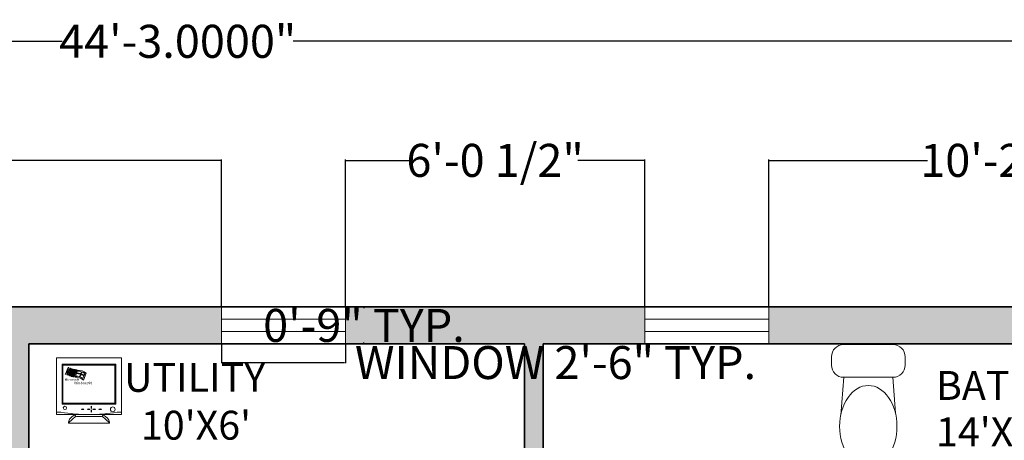
# Model space of a CAD drawing. Units: inches. Extents: x 638 to 1303, y 1 to 699.
# Tile 20 of 21: x 924 to 1163, y 597 to 699. Entities that reach past the tile are written whole.
import ezdxf

# ---------------------------------------------------------------- set-up
doc = ezdxf.new("R2010")
doc.units = ezdxf.units.IN
doc.header["$MEASUREMENT"] = 0
for name, color, linetype, lineweight in [('A-ANNO-DIMS', 2, 'Continuous', 18), ('A-AREA-IDEN', 7, 'Continuous', 18), ('A-EQPM', 8, 'Continuous', 15), ('A-EQPM-TEXT', 8, 'Continuous', 13), ('A-FLOR-FIXT', 9, 'Continuous', 18), ('A-GLAZ', 4, 'Continuous', 18), ('A-WALL', 7, 'Continuous', 35)]:
    doc.layers.add(name, color=color, linetype=linetype, lineweight=lineweight)
doc.layers.add('A-WALL-PATT', color=143, linetype='Continuous', lineweight=13, true_color=0x7aafdf)
doc.styles.add('COMPLEX', font='COMPLEX.SHX')
doc.styles.get("Standard").update_dxf_attribs({"font": 'arial.ttf'})
doc.dimstyles.get("Standard").update_dxf_attribs({"dimtxt": 8, "dimasz": 0.18, "dimexe": 0.18, "dimexo": 0.0625, "dimgap": 0.09, "dimtad": 0, "dimtih": 1, "dimtoh": 1, "dimdec": 4, "dimzin": 0, "dimdsep": 46, "dimlunit": 3, "dimtxsty": 'Standard', "dimcen": 0.09, "dimadec": 0, "dimazin": 0, "dimtfac": 1, "dimtdec": 4, "dimtofl": 0, "dimtmove": 0, "dimatfit": 3, "dimfxl": 1, "dimtolj": 1, "dimtzin": 0, "dimarcsym": 0})

# ---------------------------------------------------------------- blocks, each defined once
blk = doc.blocks.new('*D2')
at = {"layer": 'A-ANNO-DIMS', "color": 0, "lineweight": -2, "transparency": 16777216}
for p, q in [((697.24, 629.88), (697.24, 694.35)), ((697.42, 694.17), (934.76, 694.17)), ((1228.06, 694.17), (990.71, 694.17)), ((1228.24, 629.88), (1228.24, 694.35))]:
    blk.add_line(p, q, dxfattribs=at)
at = {"layer": 'A-ANNO-DIMS', "color": 0, "transparency": 16777216}
for points in [[(697.42, 694.2), (697.42, 694.14), (697.24, 694.17)], [(1228.06, 694.2), (1228.06, 694.14), (1228.24, 694.17)]]:
    blk.add_solid(points, dxfattribs=at)
at = {"layer": 'Defpoints', "color": 0, "transparency": 16777216}
for p in [(1228.24, 694.17), (697.24, 629.82), (1228.24, 629.82)]:
    blk.add_point(p, dxfattribs=at)
at = {"layer": 'A-ANNO-DIMS', "color": 0, "transparency": 16777216, "insert": (962.74, 694.17), "char_height": 8, "attachment_point": 5}
blk.add_mtext('\\A1;44\'-3.0000"', dxfattribs=at)
blk = doc.blocks.new('WIN-30')
for p, q in [((30, 9), (0, 9)), ((0, 9), (0, 0)), ((30, 0), (30, 9)), ((0, 6), (30, 6)), ((0, 3), (30, 3)), ((0, 0), (30, 0))]:
    blk.add_line(p, q)
blk = doc.blocks.new('*D24')
at = {"layer": 'A-ANNO-DIMS', "color": 0, "lineweight": -2, "transparency": 16777216}
for p, q in [((973.35, 620.76), (973.35, 616.14)), ((1003.35, 620.76), (1003.35, 616.14)), ((973.53, 616.32), (1003.17, 616.32)), ((1003.35, 616.32), (1003.53, 616.32))]:
    blk.add_line(p, q, dxfattribs=at)
at = {"layer": 'A-ANNO-DIMS', "color": 0, "transparency": 16777216}
for points in [[(973.53, 616.35), (973.53, 616.29), (973.35, 616.32)], [(1003.17, 616.35), (1003.17, 616.29), (1003.35, 616.32)]]:
    blk.add_solid(points, dxfattribs=at)
at = {"layer": 'Defpoints', "color": 0, "transparency": 16777216}
for p in [(973.35, 620.82), (1003.35, 620.82), (1003.35, 616.32)]:
    blk.add_point(p, dxfattribs=at)
at = {"layer": 'A-ANNO-DIMS', "color": 0, "transparency": 16777216, "insert": (1054.23, 616.32), "char_height": 8, "attachment_point": 5}
blk.add_mtext('\\A1;WINDOW 2\'-6" TYP.', dxfattribs=at)
blk = doc.blocks.new('*D25')
at = {"layer": 'A-ANNO-DIMS', "color": 0, "lineweight": -2, "transparency": 16777216}
for p, q in [((1003.41, 629.82), (1008.03, 629.82)), ((1007.85, 629.64), (1007.85, 629.49)), ((1003.41, 620.82), (1008.03, 620.82)), ((1007.85, 621), (1007.85, 621.14))]:
    blk.add_line(p, q, dxfattribs=at)
at = {"layer": 'A-ANNO-DIMS', "color": 0, "transparency": 16777216}
for points in [[(1007.82, 629.64), (1007.88, 629.64), (1007.85, 629.82)], [(1007.82, 621), (1007.88, 621), (1007.85, 620.82)]]:
    blk.add_solid(points, dxfattribs=at)
at = {"layer": 'Defpoints', "color": 0, "transparency": 16777216}
for p in [(1003.35, 629.82), (1007.85, 629.82), (1003.35, 620.82)]:
    blk.add_point(p, dxfattribs=at)
at = {"layer": 'A-ANNO-DIMS', "color": 0, "transparency": 16777216, "insert": (1007.85, 625.32), "char_height": 8, "attachment_point": 5}
blk.add_mtext('\\A1;0\'-9" TYP.', dxfattribs=at)
blk = doc.blocks.new('*D52')
at = {"layer": 'A-ANNO-DIMS', "color": 0, "lineweight": -2, "transparency": 16777216}
for p, q in [((793.36, 629.88), (793.36, 665.5)), ((793.54, 665.32), (869.9, 665.32)), ((973.17, 665.32), (896.8, 665.32)), ((973.35, 629.88), (973.35, 665.5))]:
    blk.add_line(p, q, dxfattribs=at)
at = {"layer": 'A-ANNO-DIMS', "color": 0, "transparency": 16777216}
for points in [[(793.54, 665.35), (793.54, 665.29), (793.36, 665.32)], [(973.17, 665.35), (973.17, 665.29), (973.35, 665.32)]]:
    blk.add_solid(points, dxfattribs=at)
at = {"layer": 'Defpoints', "color": 0, "transparency": 16777216}
for p in [(973.35, 665.32), (793.36, 629.82), (973.35, 629.82)]:
    blk.add_point(p, dxfattribs=at)
at = {"layer": 'A-ANNO-DIMS', "color": 0, "transparency": 16777216, "insert": (883.35, 665.32), "char_height": 8, "attachment_point": 5}
blk.add_mtext('\\A1;15\'-0"', dxfattribs=at)
blk = doc.blocks.new('*D53')
at = {"layer": 'A-ANNO-DIMS', "color": 0, "lineweight": -2, "transparency": 16777216}
for p, q in [((1003.35, 629.88), (1003.35, 665.5)), ((1003.53, 665.32), (1019.53, 665.32)), ((1075.67, 665.32), (1059.66, 665.32)), ((1075.85, 629.88), (1075.85, 665.5))]:
    blk.add_line(p, q, dxfattribs=at)
at = {"layer": 'A-ANNO-DIMS', "color": 0, "transparency": 16777216}
for points in [[(1003.53, 665.35), (1003.53, 665.29), (1003.35, 665.32)], [(1075.67, 665.35), (1075.67, 665.29), (1075.85, 665.32)]]:
    blk.add_solid(points, dxfattribs=at)
at = {"layer": 'Defpoints', "color": 0, "transparency": 16777216}
for p in [(1075.85, 665.32), (1003.35, 629.82), (1075.85, 629.82)]:
    blk.add_point(p, dxfattribs=at)
at = {"layer": 'A-ANNO-DIMS', "color": 0, "transparency": 16777216, "insert": (1039.6, 665.32), "char_height": 8, "attachment_point": 5}
blk.add_mtext('\\A1;6\'-0 1/2"', dxfattribs=at)
blk = doc.blocks.new('*D54')
at = {"layer": 'A-ANNO-DIMS', "color": 0, "lineweight": -2, "transparency": 16777216}
for p, q in [((1105.85, 629.88), (1105.85, 665.5)), ((1106.03, 665.32), (1144.27, 665.32)), ((1228.06, 665.32), (1189.82, 665.32)), ((1228.24, 629.88), (1228.24, 665.5))]:
    blk.add_line(p, q, dxfattribs=at)
at = {"layer": 'A-ANNO-DIMS', "color": 0, "transparency": 16777216}
for points in [[(1106.03, 665.35), (1106.03, 665.29), (1105.85, 665.32)], [(1228.06, 665.35), (1228.06, 665.29), (1228.24, 665.32)]]:
    blk.add_solid(points, dxfattribs=at)
at = {"layer": 'Defpoints', "color": 0, "transparency": 16777216}
for p in [(1228.24, 665.32), (1105.85, 629.82), (1228.24, 629.82)]:
    blk.add_point(p, dxfattribs=at)
at = {"layer": 'A-ANNO-DIMS', "color": 0, "transparency": 16777216, "insert": (1167.05, 665.32), "char_height": 8, "attachment_point": 5}
blk.add_mtext('\\A1;10\'-2 1/2"', dxfattribs=at)

msp = doc.modelspace()

# ---------------------------------------------------------------- hatches: boundary and pattern name
at = {"layer": 'A-WALL-PATT'}
h = msp.add_hatch(color=256, dxfattribs=at)
h.dxf.hatch_style = 1
h.paths.add_polyline_path([(973.34524, 629.81895), (793.35541, 629.81895), (793.35541, 620.81895), (850.23798, 620.81895), (922.23798, 620.81895), (922.23798, 524.81895), (908.94335, 524.81895), (908.94335, 520.31895), (926.73798, 520.31895), (926.73798, 544.31895), (979.3571, 544.31895), (979.3571, 548.81895), (926.73798, 548.81895), (926.73798, 620.81895), (973.34524, 620.81895)])
h.paths.add_polyline_path([(758.35541, 629.81895), (697.23798, 629.81895), (697.23798, 586.77451), (706.23798, 586.77451), (706.23798, 620.81895), (758.35541, 620.81895)])
h.paths.add_polyline_path([(1075.85281, 629.81895), (1003.34524, 629.81895), (1003.34524, 620.81895), (1046.73798, 620.81895), (1046.73798, 560.81895), (1046.73798, 548.81895), (1026.3571, 548.81895), (1026.3571, 544.31895), (1046.73798, 544.31895), (1046.73798, 486.87457), (1051.23798, 486.87457), (1051.23798, 556.31895), (1162.89753, 556.31895), (1162.89753, 560.81895), (1051.23798, 560.81895), (1051.23798, 620.81895), (1075.85281, 620.81895)])
h.paths.add_polyline_path([(1228.23798, 629.81895), (1105.85281, 629.81895), (1105.85281, 620.81895), (1219.23798, 620.81895), (1219.23798, 560.81895), (1197.89753, 560.81895), (1197.89753, 556.31895), (1219.23798, 556.31895), (1219.23798, 498.80084), (1228.23798, 498.80084)])
h.paths.add_polyline_path([(1051.23798, 439.87457), (1046.73798, 439.87457), (1046.73798, 407.81895), (1219.23798, 407.81895), (1219.23798, 381.66175), (1228.23798, 381.66175), (1228.23798, 451.80084), (1219.23798, 451.80084), (1219.23798, 412.31895), (1051.23798, 412.31895)])
h.paths.add_polyline_path([(1228.23798, 346.66175), (1219.23798, 346.66175), (1219.23798, 335.81895), (1046.73798, 335.81895), (1046.73798, 273.56895), (1051.23798, 273.56895), (1051.23798, 331.31895), (1219.23798, 331.31895), (1219.23798, 308.99654), (1228.23798, 308.99654)])
h.paths.add_polyline_path([(1228.23798, 261.99654), (1219.23798, 261.99654), (1219.23798, 211.31895), (1051.23798, 211.31895), (1051.23798, 226.56895), (1046.73798, 226.56895), (1046.73798, 211.31895), (983.84714, 211.31895), (983.84714, 206.81895), (1219.23798, 206.81895), (1219.23798, 166.83987), (1228.23798, 166.83987)])
h.paths.add_polyline_path([(1228.23798, 119.83987), (1219.23798, 119.83987), (1219.23798, 50.81895), (1197.89277, 50.81895), (1197.89277, 41.81895), (1228.23798, 41.81895)])
h.paths.add_polyline_path([(1162.89277, 50.81895), (1069.02949, 50.81895), (1069.02949, 41.81895), (1162.89277, 41.81895)])
h.paths.add_polyline_path([(1010.02949, 50.81895), (941.89631, 50.81895), (917.77455, 50.81895), (917.77455, 41.81895), (941.89631, 41.81895), (1010.02949, 41.81895)])
h.paths.add_polyline_path([(882.77455, 50.81895), (854.73798, 50.81895), (854.73798, 145.50379), (850.23798, 145.50379), (850.23798, 50.81895), (793.49755, 50.81895), (793.49755, 41.81895), (882.77455, 41.81895)])
h.paths.add_polyline_path([(746.49755, 50.81895), (706.23798, 50.81895), (706.23798, 96.57416), (697.23798, 96.57416), (697.23798, 41.81895), (746.49755, 41.81895)])
h.paths.add_polyline_path([(706.23798, 206.81895), (714.01165, 206.81895), (714.01165, 211.31895), (706.23798, 211.31895), (706.23798, 251.21966), (697.23798, 251.21966), (697.23798, 143.57416), (706.23798, 143.57416)])
h.paths.add_polyline_path([(923.84714, 211.31895), (854.73798, 211.31895), (854.73798, 397.8313), (850.23798, 397.8313), (850.23798, 388.31895), (747.9539, 388.31895), (747.9539, 383.81895), (850.23798, 383.81895), (850.23798, 311.81895), (706.23798, 311.81895), (706.23798, 342.78787), (697.23798, 342.78787), (697.23798, 281.21966), (706.23798, 281.21966), (706.23798, 307.31895), (850.23798, 307.31895), (850.23798, 211.31895), (749.01165, 211.31895), (749.01165, 206.81895), (850.23798, 206.81895), (850.23798, 192.50379), (854.73798, 192.50379), (854.73798, 206.81895), (923.84714, 206.81895)])
h.paths.add_polyline_path([(706.23798, 434.70471), (697.23798, 434.70471), (697.23798, 372.78787), (706.23798, 372.78787), (706.23798, 383.81895), (712.9539, 383.81895), (712.9539, 388.31895), (706.23798, 388.31895)])
h.paths.add_polyline_path([(706.23798, 520.31895), (850.23798, 520.31895), (850.23798, 444.8313), (854.73798, 444.8313), (854.73798, 520.31895), (861.94335, 520.31895), (861.94335, 524.81895), (706.23798, 524.81895), (706.23798, 551.77451), (697.23798, 551.77451), (697.23798, 481.70471), (706.23798, 481.70471)])

# ---------------------------------------------------------------- linework, layer by layer
at = {"layer": 'A-EQPM'}
for p, q in [((949.1339, 617.48415), (933.3859, 617.48415)), ((933.3859, 617.48415), (933.3859, 603.70465)), ((949.1339, 603.70465), (949.1339, 617.48415)), ((947.75595, 615.90935), (934.76385, 615.90935)), ((934.9607, 615.7125), (934.76385, 615.90935)), ((934.76385, 615.90935), (934.76385, 606.2637)), ((947.5591, 615.7125), (934.9607, 615.7125)), ((934.9607, 615.7125), (934.9607, 606.46055)), ((947.5591, 615.7125), (947.75595, 615.90935)), ((947.5591, 606.46055), (947.5591, 615.7125)), ((947.75595, 606.2637), (947.75595, 615.90935)), ((935.56045, 613.65093), (935.51989, 613.54356)), ((935.69184, 613.54356), (935.51989, 613.54356)), ((935.73241, 613.65093), (935.56045, 613.65093)), ((935.73241, 613.65093), (935.69184, 613.54356)), ((935.7578, 613.97034), (935.71724, 613.86298)), ((935.8892, 613.86298), (935.71724, 613.86298)), ((935.92976, 613.97034), (935.7578, 613.97034)), ((935.8593, 614.24335), (935.81874, 614.13599)), ((935.9907, 614.13599), (935.81874, 614.13599)), ((936.03126, 614.24335), (935.8593, 614.24335)), ((935.92817, 614.4156), (935.8876, 614.30824)), ((936.05956, 614.30824), (935.8876, 614.30824)), ((935.92976, 613.97034), (935.8892, 613.86298)), ((935.95694, 613.49606), (935.91131, 613.37527)), ((936.10476, 613.37527), (935.91131, 613.37527)), ((936.10012, 614.4156), (935.92817, 614.4156)), ((936.1504, 613.49606), (935.95694, 613.49606)), ((936.00602, 614.59871), (935.96545, 614.49135)), ((936.13741, 614.49135), (935.96545, 614.49135)), ((936.03126, 614.24335), (935.9907, 614.13599)), ((936.17797, 614.59871), (936.00602, 614.59871)), ((936.0924, 613.76731), (936.04677, 613.64653)), ((936.24022, 613.64653), (936.04677, 613.64653)), ((936.09289, 614.82158), (936.05233, 614.71421)), ((936.22428, 614.71421), (936.05233, 614.71421)), ((936.10012, 614.4156), (936.05956, 614.30824)), ((936.28586, 613.76731), (936.0924, 613.76731)), ((936.26485, 614.82158), (936.09289, 614.82158)), ((936.1504, 613.49606), (936.10476, 613.37527)), ((936.17797, 614.59871), (936.13741, 614.49135)), ((936.18319, 614.01116), (936.13756, 613.89038)), ((936.33101, 613.89038), (936.13756, 613.89038)), ((936.2124, 615.0804), (936.17184, 614.97304)), ((936.3438, 614.97304), (936.17184, 614.97304)), ((936.37664, 614.01116), (936.18319, 614.01116)), ((936.38436, 615.0804), (936.2124, 615.0804)), ((936.26485, 614.82158), (936.22428, 614.71421)), ((936.27496, 614.25996), (936.22933, 614.13918)), ((936.42278, 614.13918), (936.22933, 614.13918)), ((936.28586, 613.76731), (936.24022, 613.64653)), ((936.46842, 614.25996), (936.27496, 614.25996)), ((936.32591, 613.39519), (936.2752, 613.26099)), ((936.49015, 613.26099), (936.2752, 613.26099)), ((936.36139, 614.48764), (936.31576, 614.36686)), ((936.50921, 614.36686), (936.31576, 614.36686)), ((936.54085, 613.39519), (936.32591, 613.39519)), ((936.37664, 614.01116), (936.33101, 613.89038)), ((936.38436, 615.0804), (936.3438, 614.97304)), ((936.55485, 614.48764), (936.36139, 614.48764)), ((936.46161, 613.66811), (936.4109, 613.53391)), ((936.62585, 613.53391), (936.4109, 613.53391)), ((936.46842, 614.25996), (936.42278, 614.13918)), ((936.48395, 614.7278), (936.43832, 614.60702)), ((936.63177, 614.60702), (936.43832, 614.60702)), ((936.67656, 613.66811), (936.46161, 613.66811)), ((936.6774, 614.7278), (936.48395, 614.7278)), ((936.54085, 613.39519), (936.49015, 613.26099)), ((936.55485, 614.48764), (936.50921, 614.36686)), ((936.57827, 613.97664), (936.52756, 613.84244)), ((936.74251, 613.84244), (936.52756, 613.84244)), ((936.58939, 614.94132), (936.54375, 614.82054)), ((936.73721, 614.82054), (936.54375, 614.82054)), ((936.62388, 613.22892), (936.56754, 613.0798)), ((936.80637, 613.0798), (936.56754, 613.0798)), ((936.79321, 613.97664), (936.57827, 613.97664)), ((936.78284, 614.94132), (936.58939, 614.94132)), ((936.64548, 614.15895), (936.59478, 614.02475)), ((936.80972, 614.02475), (936.59478, 614.02475)), ((936.86271, 613.22892), (936.62388, 613.22892)), ((936.67656, 613.66811), (936.62585, 613.53391)), ((936.6774, 614.7278), (936.63177, 614.60702)), ((936.86043, 614.15895), (936.64548, 614.15895)), ((936.71803, 614.34659), (936.66732, 614.21239)), ((936.88227, 614.21239), (936.66732, 614.21239)), ((936.76764, 613.50791), (936.71131, 613.3588)), ((936.95014, 613.3588), (936.71131, 613.3588)), ((936.93298, 614.34659), (936.71803, 614.34659)), ((936.78284, 614.94132), (936.73721, 614.82054)), ((936.79321, 613.97664), (936.74251, 613.84244)), ((936.81588, 614.5487), (936.76517, 614.4145)), ((936.98012, 614.4145), (936.76517, 614.4145)), ((937.00647, 613.50791), (936.76764, 613.50791)), ((936.86271, 613.22892), (936.80637, 613.0798)), ((936.86043, 614.15895), (936.80972, 614.02475)), ((937.03082, 614.5487), (936.81588, 614.5487)), ((936.88103, 614.81488), (936.83033, 614.68068)), ((937.04528, 614.68068), (936.83033, 614.68068)), ((936.89189, 613.83397), (936.83555, 613.68486)), ((937.07438, 613.68486), (936.83555, 613.68486)), ((937.09598, 614.81488), (936.88103, 614.81488)), ((936.93298, 614.34659), (936.88227, 614.21239)), ((937.13072, 613.83397), (936.89189, 613.83397)), ((936.98293, 613.11024), (936.92033, 612.94456)), ((937.1857, 612.94456), (936.92033, 612.94456)), ((936.99614, 614.04392), (936.9398, 613.89481)), ((937.17863, 613.89481), (936.9398, 613.89481)), ((937.00647, 613.50791), (936.95014, 613.3588)), ((937.03082, 614.5487), (936.98012, 614.4145)), ((937.2483, 613.11024), (936.98293, 613.11024)), ((937.23497, 614.04392), (936.99614, 614.04392)), ((937.06935, 614.2598), (937.01302, 614.11069)), ((937.25185, 614.11069), (937.01302, 614.11069)), ((937.09869, 613.36808), (937.03609, 613.2024)), ((937.30146, 613.2024), (937.03609, 613.2024)), ((937.09598, 614.81488), (937.04528, 614.68068)), ((937.30819, 614.2598), (937.06935, 614.2598)), ((937.13072, 613.83397), (937.07438, 613.68486)), ((937.15261, 614.47205), (937.09628, 614.32294)), ((937.33511, 614.32294), (937.09628, 614.32294)), ((937.36406, 613.36808), (937.09869, 613.36808)), ((937.39144, 614.47205), (937.15261, 614.47205)), ((937.22397, 613.65555), (937.16138, 613.48987)), ((937.42674, 613.48987), (937.16138, 613.48987)), ((937.23322, 614.69532), (937.17689, 614.5462)), ((937.41572, 614.5462), (937.17689, 614.5462)), ((937.23497, 614.04392), (937.17863, 613.89481)), ((937.2483, 613.11024), (937.1857, 612.94456)), ((937.48934, 613.65555), (937.22397, 613.65555)), ((937.47205, 614.69532), (937.23322, 614.69532)), ((937.30819, 614.2598), (937.25185, 614.11069)), ((937.32174, 613.90278), (937.25914, 613.7371)), ((937.52451, 613.7371), (937.25914, 613.7371)), ((937.36406, 613.36808), (937.30146, 613.2024)), ((937.5871, 613.90278), (937.32174, 613.90278)), ((937.39144, 614.47205), (937.33511, 614.32294)), ((937.4113, 614.14182), (937.3487, 613.97614)), ((937.61407, 613.97614), (937.3487, 613.97614)), ((937.43288, 613.07068), (937.36332, 612.88659)), ((937.65818, 612.88659), (937.36332, 612.88659)), ((937.67667, 614.14182), (937.4113, 614.14182)), ((937.47205, 614.69532), (937.41572, 614.5462)), ((937.48934, 613.65555), (937.42674, 613.48987)), ((937.72773, 613.07068), (937.43288, 613.07068)), ((937.51777, 614.37356), (937.45518, 614.20788)), ((937.72054, 614.20788), (937.45518, 614.20788)), ((937.53239, 613.32808), (937.46284, 613.14399)), ((937.75769, 613.14399), (937.46284, 613.14399)), ((937.78314, 614.37356), (937.51777, 614.37356)), ((937.5871, 613.90278), (937.52451, 613.7371)), ((937.82725, 613.32808), (937.53239, 613.32808)), ((937.61473, 614.61999), (937.55213, 614.45431)), ((937.8175, 614.45431), (937.55213, 614.45431)), ((937.62605, 613.54452), (937.5565, 613.36043)), ((937.85136, 613.36043), (937.5565, 613.36043)), ((937.67667, 614.14182), (937.61407, 613.97614)), ((937.8801, 614.61999), (937.61473, 614.61999)), ((937.92091, 613.54452), (937.62605, 613.54452)), ((937.71825, 613.79461), (937.6487, 613.61052)), ((937.94356, 613.61052), (937.6487, 613.61052)), ((937.72773, 613.07068), (937.65818, 612.88659)), ((938.01311, 613.79461), (937.71825, 613.79461)), ((937.78314, 614.37356), (937.72054, 614.20788)), ((937.81777, 614.052), (937.74822, 613.86791)), ((938.04307, 613.86791), (937.74822, 613.86791)), ((937.82725, 613.32808), (937.75769, 613.14399)), ((937.8801, 614.61999), (937.8175, 614.45431)), ((938.11262, 614.052), (937.81777, 614.052)), ((937.91143, 614.26845), (937.84188, 614.08436)), ((938.13674, 614.08436), (937.84188, 614.08436)), ((937.92091, 613.54452), (937.85136, 613.36043)), ((938.5065, 614.4536), (937.88264, 612.8023)), ((938.20629, 614.26845), (937.91143, 614.26845)), ((938.01095, 614.52584), (937.9414, 614.34175)), ((938.23625, 614.34175), (937.9414, 614.34175)), ((938.01311, 613.79461), (937.94356, 613.61052)), ((938.3058, 614.52584), (938.01095, 614.52584)), ((938.11262, 614.052), (938.04307, 613.86791)), ((938.20629, 614.26845), (938.13674, 614.08436)), ((938.3058, 614.52584), (938.23625, 614.34175)), ((939.21122, 613.49849), (938.98127, 612.88984)), ((939.34883, 613.45242), (939.11873, 612.8434)), ((939.43496, 614.09069), (939.25994, 613.62745)), ((939.5719, 614.04285), (939.39696, 613.57982)), ((940.033, 613.10177), (939.80214, 612.49075)), ((940.55577, 613.72496), (939.93478, 612.0813)), ((940.25246, 613.68264), (940.07795, 613.22076)), ((934.9607, 606.46055), (934.76385, 606.2637)), ((934.76385, 606.33758), (947.75595, 606.33758)), ((934.76385, 606.2637), (947.75595, 606.2637)), ((934.9607, 606.46055), (947.5591, 606.46055)), ((947.5591, 606.46055), (947.75595, 606.2637)), ((933.3859, 604.28873), (934.46955, 604.28873)), ((933.3859, 603.70465), (949.1339, 603.70465)), ((936.31387, 601.69384), (938.07136, 603.31625)), ((938.00659, 603.70465), (938.00659, 603.46222)), ((938.20344, 603.26537), (944.31636, 603.26537)), ((946.20593, 601.69384), (944.44844, 603.31625)), ((944.51321, 603.70465), (944.51321, 603.46222)), ((949.1339, 604.28873), (948.05025, 604.28873)), ((936.47276, 601.61318), (946.04704, 601.61318))]:
    msp.add_line(p, q, dxfattribs=at)
for centre, radius in [((935.43024, 605.31291), 0.40333), ((947.01379, 604.98036), 0.57591)]:
    msp.add_circle(centre, radius, dxfattribs=at)
for centre, radius, start, end in [((937.95822, 609.76839), 3.04243, 49.4835836, 91.3691071), ((938.07648, 609.98506), 3.04243, 55.4448091, 92.0627886), ((938.31437, 610.59126), 3.04243, 72.8555578, 92.2323881), ((938.32987, 610.73067), 3.04243, 72.1996997, 91.523266), ((938.50037, 611.19536), 3.04243, 54.8384352, 91.4269699), ((938.57921, 611.41204), 3.04243, 49.4835836, 91.3695198), ((938.31437, 610.59126), 3.04243, 55.6055903, 70.1225489), ((938.32987, 610.73067), 3.04243, 54.9306221, 69.4677052), ((941.2599, 643.46835), 39.7637, 260.1675485, 279.8324515), ((938.20344, 603.46222), 0.19685, 180, 270), ((944.31636, 603.46222), 0.19685, 270, 0), ((936.47276, 601.81003), 0.19685, 162.3544458, 270), ((946.04704, 601.81003), 0.19685, 270, 17.6455542)]:
    msp.add_arc(centre, radius, start, end, dxfattribs=at)
for centre, major_axis in [((941.83551, 605.48033), (0, 0.2961)), ((939.75314, 605.02038), (0.2961, 0)), ((941.19297, 605.02038), (0.2961, 0)), ((942.52038, 605.02038), (0.2961, 0)), ((943.97679, 605.02038), (0.2961, 0))]:
    msp.add_ellipse(centre, major_axis=major_axis, ratio=0.192174607, dxfattribs=at)
at = {"layer": 'A-EQPM', "extrusion": (0, 0, -1)}
msp.add_ellipse((941.83551, 604.56043), major_axis=(0, -0.2961), ratio=0.192174607, dxfattribs=at)
at = {"layer": 'A-EQPM'}
for points in [[(937.96953, 603.70465), (936.73258, 602.92887), (936.50088, 602.49751), (936.33796, 602.03566), (936.28517, 601.86971)], [(944.55027, 603.70465), (945.78722, 602.92887), (946.01892, 602.49751), (946.18184, 602.03566), (946.23463, 601.86971)]]:
    msp.add_open_spline(points, degree=3, knots=[24.378192663, 24.378192663, 24.378192663, 24.378192663, 48.535416358, 61.80523206, 61.80523206, 61.80523206, 61.80523206], dxfattribs=at)
at = {"layer": 'A-FLOR-FIXT'}
for p, q in [((1124.02103, 620.67354), (1135.91726, 620.67354)), ((1121.04698, 615.71678), (1121.04698, 617.69949)), ((1138.89132, 617.69949), (1138.89132, 615.71678)), ((1124.02103, 612.74272), (1123.30242, 603.59844)), ((1135.91726, 612.74272), (1124.02103, 612.74272)), ((1135.91726, 612.74272), (1136.54063, 604.03186))]:
    msp.add_line(p, q, dxfattribs=at)
for centre, start, end in [((1124.02103, 617.69949), 90, 180), ((1135.91726, 617.69949), 0, 90), ((1124.02103, 615.71678), 180, 270), ((1135.91726, 615.71678), 270, 0)]:
    msp.add_arc(centre, 2.97406, start, end, dxfattribs=at)
msp.add_ellipse((1129.96915, 600.8465), major_axis=(0, -9.91352), ratio=0.7, dxfattribs=at)
at = {"layer": 'A-WALL'}
for p, q in [((1228.23798, 629.81895), (697.23798, 629.81895)), ((1046.73798, 620.81895), (926.73798, 620.81895)), ((926.73798, 548.81895), (926.73798, 620.81895)), ((1046.73798, 620.81895), (1046.73798, 560.81895)), ((1219.23798, 620.81895), (1051.23798, 620.81895)), ((1051.23798, 620.81895), (1051.23798, 560.81895))]:
    msp.add_line(p, q, dxfattribs=at)

# ---------------------------------------------------------------- block references
at = {"layer": 'A-GLAZ'}
for p in [(973.34542, 620.819), (1075.853, 620.819)]:
    msp.add_blockref('WIN-30', p, dxfattribs=at)

# ---------------------------------------------------------------- texts
at = {"layer": 'A-AREA-IDEN'}
for s, p in [('UTILITY', (949.7603, 609.23113)), ('BATH ROOM', (1146.35423, 607.27456)), ("10'X6'", (953.83873, 597.63286)), ("14'X5'", (1146.35423, 596.02968))]:
    msp.add_text(s, height=7, dxfattribs=at).set_placement(p)
at = {"layer": 'A-EQPM-TEXT', "extrusion": (0, 0, -1), "style": 'COMPLEX', "text_generation_flag": 2}
for s, p in [('Microsoft', (-935.36318, 611.90088)), ('Windows98', (-937.71286, 611.06692))]:
    msp.add_text(s, height=0.59055, dxfattribs=at).set_placement(p)

# ---------------------------------------------------------------- dimensions: what is measured, and where the dimension line sits
at = {"layer": 'A-ANNO-DIMS'}
for base, p1, p2, override, picture, middle in [((1228.23798, 694.16557), (697.23798, 629.81895), (1228.23798, 629.81895), {"dimclrd": 0, "dimclre": 0, "dimclrt": 0}, '*D2', (962.73798, 694.16557)), ((1075.85281, 665.31895), (1003.34524, 629.81895), (1075.85281, 629.81895), {"dimdec": 1, "dimlfac": 1, "dimrnd": 0, "dimzin": 1, "dimdsep": 46, "dimlunit": 4, "dimfrac": 2}, '*D53', (1039.59902, 665.31895)), ((1228.23798, 665.31895), (1105.85281, 629.81895), (1228.23798, 629.81895), {"dimdec": 1, "dimlfac": 1, "dimrnd": 0, "dimzin": 1, "dimdsep": 46, "dimlunit": 4, "dimfrac": 2}, '*D54', (1167.0454, 665.31895)), ((973.34524, 665.31895), (793.35541, 629.81895), (973.34524, 629.81895), {"dimdec": 1, "dimlfac": 1, "dimrnd": 0, "dimzin": 1, "dimdsep": 46, "dimlunit": 4, "dimfrac": 2}, '*D52', (883.35032, 665.31895))]:
    dim = msp.add_linear_dim(base=base, p1=p1, p2=p2, dimstyle='Standard', override=override, dxfattribs=at)
    dim.commit()
    dim.dimension.update_dxf_attribs({"geometry": picture, "text_midpoint": middle})
dim = msp.add_linear_dim(base=(1007.84524, 629.81895), p1=(1003.34524, 620.81895), p2=(1003.34524, 629.81895), angle=90, text='<> TYP.', dimstyle='Standard', override={"dimdec": 1, "dimlfac": 1, "dimrnd": 0, "dimzin": 1, "dimdsep": 46, "dimlunit": 4, "dimfrac": 2}, dxfattribs=at)
dim.commit()
dim.dimension.update_dxf_attribs({"geometry": '*D25', "text_midpoint": (1007.84524, 625.31895)})
dim = msp.add_linear_dim(base=(1003.34524, 616.31895), p1=(973.34524, 620.81895), p2=(1003.34524, 620.81895), text='WINDOW <> TYP.', dimstyle='Standard', override={"dimdec": 1, "dimlfac": 1, "dimrnd": 0, "dimzin": 1, "dimdsep": 46, "dimlunit": 4, "dimfrac": 2}, dxfattribs=at)
dim.commit()
dim.dimension.update_dxf_attribs({"geometry": '*D24', "text_midpoint": (1054.23188, 616.31895)})

doc.saveas('drawing.dxf')
